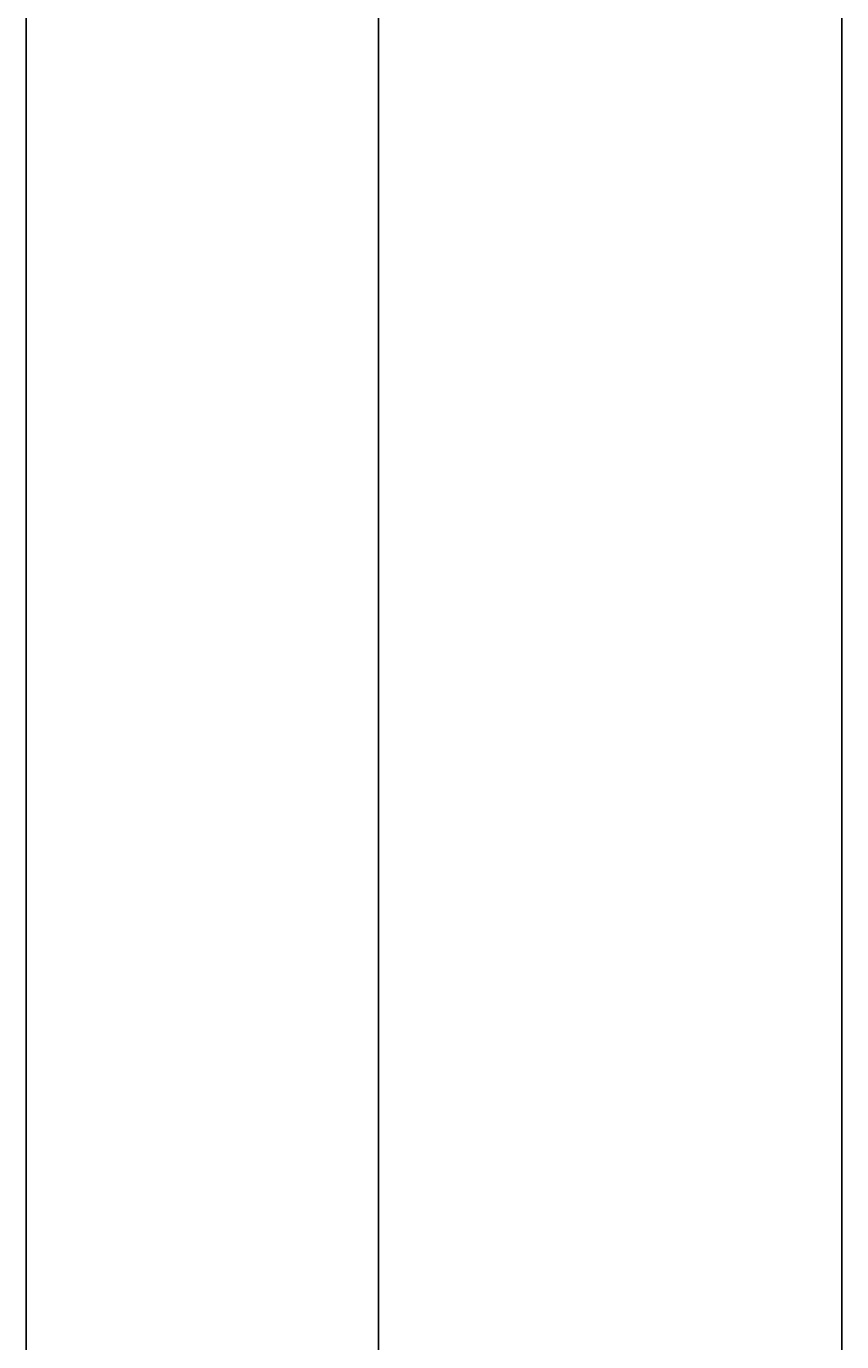
# Model space of a CAD drawing. Units: inches. Extents: x 1601 to 2297, y 1496 to 2631.
# Tile 5 of 57: x 1601 to 1686, y 1835 to 1973. Entities that reach past the tile are written whole.
import ezdxf

# ---------------------------------------------------------------- set-up
doc = ezdxf.new("R2010")
doc.units = ezdxf.units.IN
doc.layers.add('A-ANNO-DIMS', color=2, linetype='Continuous', lineweight=18)
doc.layers.add('A-ANNO-TTLB', color=7, linetype='Continuous', lineweight=25)
doc.styles.get("Standard").update_dxf_attribs({"font": 'arial.ttf'})
doc.dimstyles.get("Standard").update_dxf_attribs({"dimtxt": 0.18, "dimasz": 0.18, "dimexe": 0.18, "dimexo": 0.0625, "dimgap": 0.09, "dimtad": 0, "dimtih": 1, "dimtoh": 1, "dimdec": 4, "dimzin": 0, "dimdsep": 46, "dimtxsty": 'Standard', "dimcen": 0.09, "dimadec": 0, "dimazin": 0, "dimtfac": 1, "dimtdec": 4, "dimtofl": 0, "dimtmove": 0, "dimatfit": 3, "dimfxl": 1, "dimtolj": 1, "dimtzin": 0, "dimarcsym": 0})

# ---------------------------------------------------------------- blocks, each defined once
blk = doc.blocks.new('*D30')
at = {"layer": 'A-ANNO-DIMS', "color": 0, "lineweight": -2, "transparency": 16777216}
for p, q in [((1685.97, 2031.33), (1637.31, 2031.33)), ((1637.49, 2031.15), (1637.49, 1833.51)), ((1637.49, 1635.51), (1637.49, 1833.14)), ((1685.97, 1635.33), (1637.31, 1635.33))]:
    blk.add_line(p, q, dxfattribs=at)
at = {"layer": 'A-ANNO-DIMS', "color": 0, "transparency": 16777216}
for points in [[(1637.46, 2031.15), (1637.52, 2031.15), (1637.49, 2031.33)], [(1637.46, 1635.51), (1637.52, 1635.51), (1637.49, 1635.33)]]:
    blk.add_solid(points, dxfattribs=at)
at = {"layer": 'Defpoints', "color": 0, "transparency": 16777216}
for p in [(1637.49, 2031.33), (1686.04, 2031.33), (1686.04, 1635.33)]:
    blk.add_point(p, dxfattribs=at)
at = {"layer": 'A-ANNO-DIMS', "color": 0, "transparency": 16777216, "insert": (1637.49, 1833.33), "char_height": 0.18, "attachment_point": 5}
blk.add_mtext('\\A1;396', dxfattribs=at)
blk = doc.blocks.new('*D36')
at = {"layer": 'A-ANNO-DIMS', "color": 0, "lineweight": -2, "transparency": 16777216}
for p, q in [((1686.04, 1635.39), (1686.04, 2581.06)), ((1686.22, 2580.88), (1712.36, 2580.88)), ((1739.15, 2580.88), (1713.01, 2580.88)), ((1739.33, 1635.39), (1739.33, 2581.06))]:
    blk.add_line(p, q, dxfattribs=at)
at = {"layer": 'A-ANNO-DIMS', "color": 0, "transparency": 16777216}
for points in [[(1686.22, 2580.91), (1686.22, 2580.85), (1686.04, 2580.88)], [(1739.15, 2580.91), (1739.15, 2580.85), (1739.33, 2580.88)]]:
    blk.add_solid(points, dxfattribs=at)
at = {"layer": 'Defpoints', "color": 0, "transparency": 16777216}
for p in [(1739.33, 2580.88), (1686.04, 1635.33), (1739.33, 1635.33)]:
    blk.add_point(p, dxfattribs=at)
at = {"layer": 'A-ANNO-DIMS', "color": 0, "transparency": 16777216, "insert": (1712.69, 2580.88), "char_height": 0.18, "attachment_point": 5}
blk.add_mtext('\\A1;53.3', dxfattribs=at)

msp = doc.modelspace()

# ---------------------------------------------------------------- linework, layer by layer
at = {"layer": 'A-ANNO-TTLB'}
msp.add_lwpolyline([(1600.5933, 2631.1477), (2297.129, 2631.1477), (2297.129, 1496.1026), (1600.5933, 1496.1026)], close=True, dxfattribs=at)

# ---------------------------------------------------------------- dimensions: what is measured, and where the dimension line sits
at = {"layer": 'A-ANNO-DIMS'}
dim = msp.add_linear_dim(base=(1739.3335, 2580.8754), p1=(1686.0373, 1635.3254), p2=(1739.3335, 1635.3254), dimstyle='Standard', override={"dimdec": 1, "dimlfac": 1, "dimrnd": 0, "dimzin": 0, "dimdsep": 46, "dimlunit": 2}, dxfattribs=at)
dim.commit()
dim.dimension.update_dxf_attribs({"geometry": '*D36', "text_midpoint": (1712.6854, 2580.8754)})
dim = msp.add_linear_dim(base=(1637.4873, 2031.3254), p1=(1686.0373, 1635.3254), p2=(1686.0373, 2031.3254), angle=90, dimstyle='Standard', override={"dimdec": 0, "dimlfac": 1, "dimrnd": 0, "dimzin": 0, "dimdsep": 46, "dimlunit": 2}, dxfattribs=at)
dim.commit()
dim.dimension.update_dxf_attribs({"geometry": '*D30', "text_midpoint": (1637.4873, 1833.3254)})

doc.saveas('drawing.dxf')
